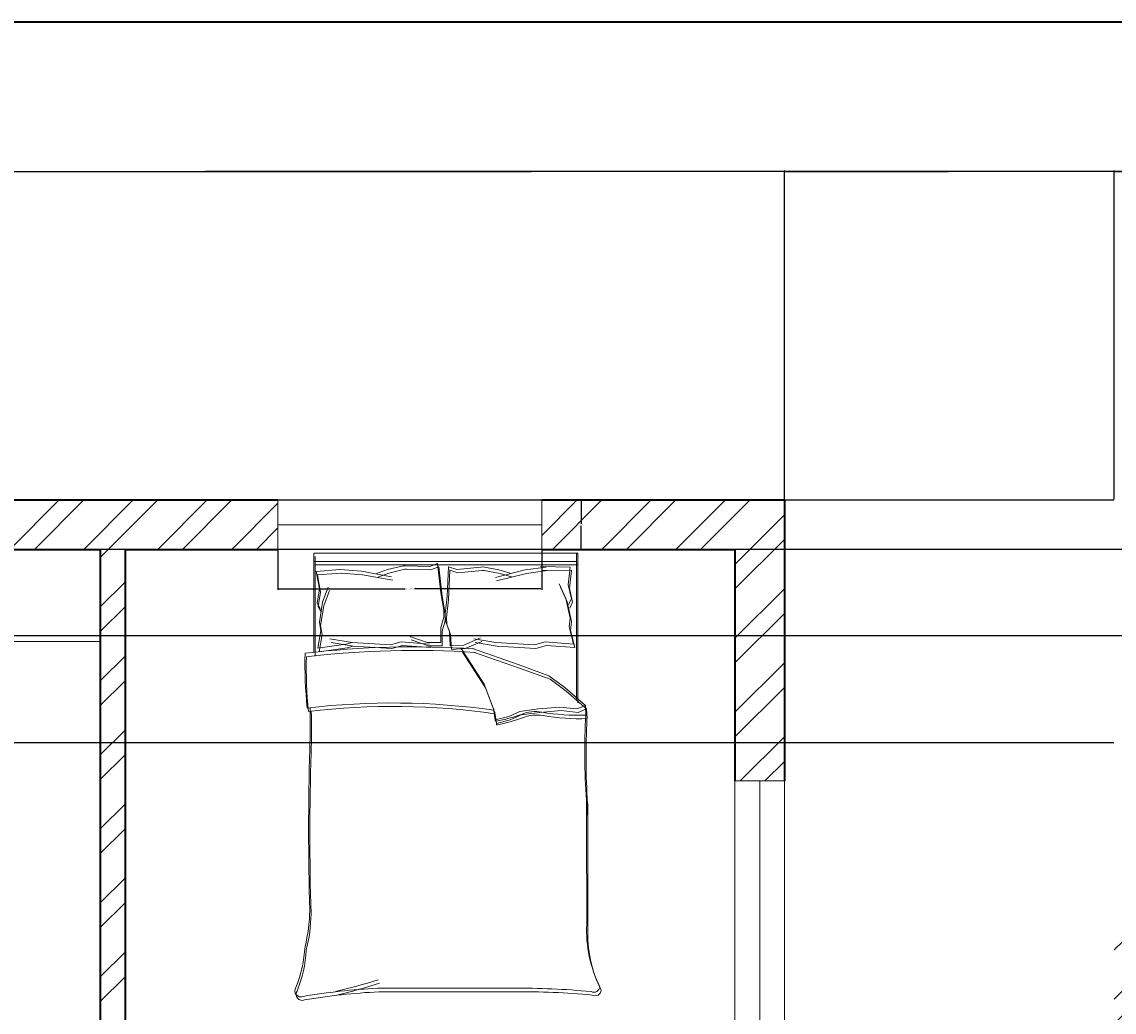
# Model space of a CAD drawing. Units: inches. Extents: x 2552 to 3217, y 1417 to 2737.
# Tile 19 of 25: x 2710 to 2909, y 2556 to 2737. Entities that reach past the tile are written whole.
import ezdxf

# ---------------------------------------------------------------- set-up
doc = ezdxf.new("R2010")
doc.units = ezdxf.units.IN
for name, color, linetype, lineweight in [('A-ANNO-DIMS', 2, 'Continuous', 18), ('A-ANNO-TTLB', 7, 'Continuous', 35), ('A-FLOR-CASE', 9, 'Continuous', 18), ('A-FURN', 8, 'Continuous', 13), ('A-GLAZ', 161, 'Continuous', 18), ('A-WALL', 7, 'Continuous', 35), ('A-WALL-PATT', 217, 'Continuous', 13)]:
    doc.layers.add(name, color=color, linetype=linetype, lineweight=lineweight)
doc.styles.get("Standard").update_dxf_attribs({"font": 'arial.ttf'})
doc.dimstyles.get("Standard").update_dxf_attribs({"dimtxt": 0.18, "dimasz": 0.18, "dimexe": 0.18, "dimexo": 0.0625, "dimgap": 0.09, "dimtad": 0, "dimtih": 1, "dimtoh": 1, "dimdec": 4, "dimzin": 0, "dimdsep": 46, "dimtxsty": 'Standard', "dimcen": 0.09, "dimadec": 0, "dimazin": 0, "dimtfac": 1, "dimtdec": 4, "dimtofl": 0, "dimtmove": 0, "dimatfit": 3, "dimfxl": 1, "dimtolj": 1, "dimtzin": 0, "dimarcsym": 0})

# ---------------------------------------------------------------- blocks, each defined once
blk = doc.blocks.new('BED-DOUBLE')
for p, q in [((3.47, 63.33), (3.47, 81.44)), ((3.47, 81.44), (51.49, 81.44)), ((3.47, 79.91), (51.27, 79.91)), ((3.48, 63.33), (3.48, 81.44)), ((3.48, 79.91), (51.27, 79.91)), ((3.7, 62.69), (3.7, 80.8)), ((3.7, 62.69), (3.7, 80.8)), ((24.54, 78.99), (25.98, 79.57)), ((24.54, 78.99), (25.98, 79.57)), ((25.98, 79.57), (26.56, 74.22)), ((25.98, 79.57), (26.56, 74.22)), ((51.27, 81.44), (51.27, 54.83)), ((51.27, 81.44), (51.27, 54.83)), ((51.49, 81.44), (51.49, 80.8)), ((51.49, 80.8), (51.49, 54.19)), ((51.49, 80.8), (51.49, 54.19)), ((3.7, 79.27), (51.49, 79.27)), ((3.7, 79.27), (51.49, 79.27)), ((3.89, 78.13), (4.47, 74.95)), ((3.89, 78.13), (4.47, 74.95)), ((3.9, 78.11), (8.18, 78.43)), ((3.9, 78.11), (8.18, 78.43)), ((4.13, 77.47), (8.41, 77.8)), ((4.13, 77.47), (8.41, 77.8)), ((8.18, 78.43), (8.28, 78.42)), ((8.18, 78.43), (8.28, 78.42)), ((8.28, 78.42), (12.11, 78.13)), ((8.28, 78.42), (12.11, 78.13)), ((8.41, 77.8), (8.51, 77.78)), ((8.41, 77.8), (8.51, 77.78)), ((8.51, 77.78), (12.34, 77.49)), ((8.51, 77.78), (12.34, 77.49)), ((12.11, 78.13), (17.6, 77.12)), ((12.11, 78.13), (17.6, 77.12)), ((14.85, 77.69), (16.88, 78.42)), ((14.85, 77.69), (16.88, 78.42)), ((15.08, 77.05), (17.11, 77.78)), ((15.08, 77.05), (17.11, 77.78)), ((16.88, 78.42), (19.77, 79.14)), ((16.88, 78.42), (19.77, 79.14)), ((17.11, 77.78), (20, 78.5)), ((17.11, 77.78), (20, 78.5)), ((19.77, 79.14), (20.09, 79.14)), ((19.77, 79.14), (20.09, 79.14)), ((20, 78.5), (20.32, 78.5)), ((20, 78.5), (20.32, 78.5)), ((20.09, 79.14), (24.54, 78.99)), ((20.09, 79.14), (24.54, 78.99)), ((20.32, 78.5), (24.77, 78.36)), ((20.32, 78.5), (24.77, 78.36)), ((24.77, 78.36), (26.21, 78.93)), ((24.77, 78.36), (26.21, 78.93)), ((26.21, 78.93), (26.79, 73.58)), ((26.21, 78.93), (26.79, 73.58)), ((27.98, 78.95), (27.73, 73.58)), ((27.98, 78.95), (27.73, 73.58)), ((28.21, 78.31), (27.96, 72.94)), ((28.21, 78.31), (27.96, 72.94)), ((29.46, 78.46), (27.98, 78.95)), ((29.46, 78.46), (27.98, 78.95)), ((29.68, 77.83), (28.21, 78.31)), ((29.68, 77.83), (28.21, 78.31)), ((33.88, 78.89), (29.46, 78.46)), ((33.88, 78.89), (29.46, 78.46)), ((34.11, 78.25), (29.68, 77.83)), ((34.11, 78.25), (29.68, 77.83)), ((34.2, 78.91), (33.88, 78.89)), ((34.2, 78.91), (33.88, 78.89)), ((34.43, 78.27), (34.11, 78.25)), ((34.43, 78.27), (34.11, 78.25)), ((37.14, 78.36), (34.2, 78.91)), ((37.14, 78.36), (34.2, 78.91)), ((37.36, 77.73), (34.43, 78.27)), ((37.36, 77.73), (34.43, 78.27)), ((41.91, 78.37), (36.49, 77.02)), ((41.91, 78.37), (36.5, 77.02)), ((42.14, 77.73), (36.72, 76.38)), ((42.14, 77.73), (36.72, 76.38)), ((39.2, 77.77), (37.14, 78.36)), ((39.2, 77.77), (37.14, 78.36)), ((39.43, 77.13), (37.36, 77.73)), ((39.43, 77.13), (37.36, 77.73)), ((45.71, 78.9), (41.91, 78.37)), ((45.71, 78.9), (41.91, 78.37)), ((45.94, 78.26), (42.14, 77.73)), ((45.94, 78.26), (42.14, 77.73)), ((50.11, 78.89), (44.71, 78.98)), ((44.71, 78.98), (45.71, 78.9)), ((50.11, 78.89), (44.71, 78.98)), ((44.71, 78.98), (45.71, 78.9)), ((50.34, 78.25), (44.94, 78.34)), ((44.94, 78.34), (45.94, 78.26)), ((50.34, 78.25), (44.94, 78.34)), ((44.94, 78.34), (45.94, 78.26)), ((50.11, 78.89), (49.73, 75.68)), ((50.11, 78.89), (49.73, 75.68)), ((50.34, 78.25), (49.96, 75.04)), ((50.34, 78.25), (49.96, 75.04)), ((4.12, 77.49), (4.7, 74.31)), ((4.12, 77.49), (4.7, 74.31)), ((12.34, 77.49), (17.83, 76.48)), ((12.34, 77.49), (17.83, 76.48)), ((49.31, 73.19), (48.13, 75.86)), ((49.31, 73.19), (48.13, 75.86)), ((49.73, 75.68), (50.33, 73.1)), ((49.73, 75.68), (50.33, 73.1)), ((4.47, 74.95), (4.04, 72.34)), ((4.47, 74.95), (4.04, 72.34)), ((4.7, 74.31), (4.27, 71.7)), ((4.7, 74.31), (4.27, 71.7)), ((5.05, 72.49), (6.06, 75.24)), ((5.05, 72.49), (6.06, 75.24)), ((5.28, 71.85), (6.29, 74.6)), ((5.28, 71.85), (6.29, 74.6)), ((26.56, 74.22), (27.14, 71.04)), ((26.56, 74.22), (27.14, 71.04)), ((26.79, 73.58), (27.37, 70.4)), ((26.79, 73.58), (27.37, 70.4)), ((27.73, 73.58), (27.35, 70.37)), ((27.73, 73.58), (27.35, 70.37)), ((49.54, 72.55), (48.36, 75.23)), ((49.54, 72.55), (48.36, 75.23)), ((49.96, 75.04), (50.56, 72.47)), ((49.96, 75.04), (50.56, 72.47)), ((4.04, 72.34), (4.62, 71.33)), ((4.04, 72.34), (4.62, 71.33)), ((4.27, 71.7), (4.85, 70.69)), ((4.27, 71.7), (4.85, 70.69)), ((4.47, 68.87), (5.05, 72.49)), ((4.47, 68.87), (5.05, 72.49)), ((4.7, 68.23), (5.28, 71.85)), ((4.7, 68.23), (5.28, 71.85)), ((27.96, 72.94), (27.58, 69.73)), ((27.96, 72.94), (27.58, 69.73)), ((50.11, 69.61), (49.31, 73.19)), ((50.11, 69.61), (49.31, 73.19)), ((50.34, 68.98), (49.54, 72.55)), ((50.34, 68.98), (49.54, 72.55)), ((50.33, 73.1), (49.81, 72.06)), ((50.33, 73.1), (49.81, 72.06)), ((50.56, 72.47), (50.04, 71.42)), ((50.56, 72.47), (50.04, 71.42)), ((27.14, 69.74), (26.56, 67.86)), ((27.14, 69.74), (26.56, 67.86)), ((27.14, 71.04), (27.14, 69.74)), ((27.14, 71.04), (27.14, 69.74)), ((27.35, 70.37), (27.44, 69.07)), ((27.35, 70.37), (27.44, 69.07)), ((27.37, 70.4), (27.37, 69.1)), ((27.37, 70.4), (27.37, 69.1)), ((27.58, 69.73), (27.66, 68.43)), ((27.58, 69.73), (27.66, 68.43)), ((49.92, 68.01), (50.11, 69.61)), ((49.92, 68.01), (50.11, 69.61)), ((4.76, 67.28), (4.47, 68.87)), ((4.76, 67.28), (4.47, 68.87)), ((4.99, 66.64), (4.7, 68.23)), ((4.99, 66.64), (4.7, 68.23)), ((26.56, 67.86), (26.56, 65.18)), ((26.56, 67.86), (26.56, 65.18)), ((27.37, 69.1), (26.79, 67.22)), ((27.37, 69.1), (26.79, 67.22)), ((27.44, 69.07), (28.13, 67.23)), ((27.44, 69.07), (28.13, 67.23)), ((27.66, 68.43), (28.36, 66.59)), ((27.66, 68.43), (28.36, 66.59)), ((50.7, 64.87), (49.92, 68.01)), ((50.7, 64.87), (49.92, 68.01)), ((50.15, 67.37), (50.34, 68.98)), ((50.15, 67.37), (50.34, 68.98)), ((4.18, 64.1), (4.76, 67.28)), ((4.18, 64.1), (4.76, 67.28)), ((4.41, 63.46), (4.99, 66.64)), ((4.41, 63.46), (4.99, 66.64)), ((6.38, 65.81), (10.41, 65.15)), ((6.38, 65.81), (10.41, 65.15)), ((24.1, 65.18), (20.96, 66.27)), ((24.1, 65.18), (20.96, 66.27)), ((24.33, 64.54), (21.19, 65.63)), ((24.33, 64.54), (21.19, 65.63)), ((26.79, 67.22), (26.79, 64.54)), ((26.79, 67.22), (26.79, 64.54)), ((28.13, 67.23), (28.3, 64.55)), ((28.13, 67.23), (28.3, 64.55)), ((28.36, 66.59), (28.53, 63.91)), ((28.36, 66.59), (28.53, 63.91)), ((30.75, 64.7), (33.82, 65.99)), ((30.75, 64.7), (33.82, 65.99)), ((32.56, 65.81), (36.6, 65.15)), ((32.56, 65.81), (36.6, 65.15)), ((50.93, 64.23), (50.15, 67.37)), ((50.93, 64.23), (50.15, 67.37)), ((9.28, 64.83), (4.18, 64.1)), ((9.28, 64.83), (4.18, 64.1)), ((9.51, 64.19), (4.41, 63.46)), ((9.51, 64.19), (4.41, 63.46)), ((6.61, 65.18), (10.64, 64.51)), ((6.61, 65.18), (10.64, 64.51)), ((10.41, 65.15), (9.28, 64.83)), ((10.41, 65.15), (9.28, 64.83)), ((10.64, 64.51), (9.51, 64.19)), ((10.64, 64.51), (9.51, 64.19)), ((10.41, 65.15), (17.42, 64.72)), ((10.41, 65.15), (17.42, 64.72)), ((10.64, 64.51), (17.65, 64.08)), ((10.64, 64.51), (17.65, 64.08)), ((17.42, 64.72), (19.38, 65.27)), ((17.42, 64.72), (19.38, 65.27)), ((17.65, 64.08), (19.61, 64.63)), ((17.65, 64.08), (19.61, 64.63)), ((19.38, 65.27), (24.52, 64.87)), ((19.38, 65.27), (24.52, 64.87)), ((19.61, 64.63), (24.74, 64.23)), ((19.61, 64.63), (24.74, 64.23)), ((26.56, 65.18), (24.1, 65.18)), ((26.56, 65.18), (24.1, 65.18)), ((26.79, 64.54), (24.33, 64.54)), ((26.79, 64.54), (24.33, 64.54)), ((28.3, 64.55), (30.75, 64.7)), ((28.3, 64.55), (30.75, 64.7)), ((28.53, 63.91), (30.98, 64.06)), ((28.53, 63.91), (30.98, 64.06)), ((30.26, 64.06), (34.45, 57.57)), ((30.26, 64.06), (34.45, 57.57)), ((30.98, 64.06), (34.05, 65.35)), ((30.98, 64.06), (34.05, 65.35)), ((40.64, 61.13), (32.31, 64.06)), ((40.64, 61.13), (32.31, 64.06)), ((32.79, 65.18), (36.82, 64.51)), ((32.79, 65.18), (36.82, 64.51)), ((36.6, 65.15), (43.61, 64.72)), ((36.6, 65.15), (43.61, 64.72)), ((36.82, 64.51), (43.83, 64.08)), ((36.82, 64.51), (43.83, 64.08)), ((43.61, 64.72), (45.57, 65.27)), ((43.61, 64.72), (45.57, 65.27)), ((43.83, 64.08), (45.79, 64.63)), ((43.83, 64.08), (45.79, 64.63)), ((45.57, 65.27), (50.7, 64.87)), ((45.57, 65.27), (50.7, 64.87)), ((45.79, 64.63), (50.93, 64.23)), ((45.79, 64.63), (50.93, 64.23)), ((30.49, 63.42), (34.68, 56.93)), ((30.49, 63.42), (34.68, 56.93)), ((40.87, 60.49), (32.53, 63.42)), ((40.87, 60.49), (32.53, 63.42)), ((46.22, 59.11), (40.64, 61.13)), ((46.22, 59.11), (40.64, 61.13)), ((46.45, 58.48), (40.87, 60.49)), ((46.45, 58.48), (40.87, 60.49)), ((49.16, 56.95), (46.22, 59.11)), ((49.16, 56.95), (46.22, 59.11)), ((49.39, 56.31), (46.45, 58.48)), ((49.39, 56.31), (46.45, 58.48)), ((34.45, 57.57), (36.15, 53.08)), ((34.45, 57.57), (36.15, 53.08)), ((34.68, 56.93), (36.38, 52.44)), ((34.68, 56.93), (36.38, 52.44)), ((52.87, 53.7), (49.16, 56.95)), ((52.87, 53.7), (49.16, 56.95)), ((53.1, 53.06), (49.39, 56.31)), ((53.1, 53.06), (49.39, 56.31)), ((51.33, 53.08), (52.87, 53.7)), ((51.33, 53.08), (52.87, 53.7)), ((52.95, 51.95), (52.87, 53.7, 3.87)), ((52.95, 51.95), (52.87, 53.7, 3.87)), ((36.15, 53.08), (36.46, 51.07)), ((36.15, 53.08), (36.46, 51.07)), ((36.38, 52.44), (36.69, 50.43)), ((36.38, 52.44), (36.69, 50.43)), ((36.46, 51.07), (38.94, 51.69)), ((36.46, 51.07), (38.94, 51.69)), ((38.94, 51.69), (40.95, 52.61)), ((38.94, 51.69), (40.95, 52.61)), ((39.17, 51.05), (41.18, 51.97)), ((39.17, 51.05), (41.18, 51.97)), ((40.95, 52.61), (44.36, 53.08)), ((40.95, 52.61), (44.36, 53.08)), ((41.18, 51.97), (44.59, 52.44)), ((41.18, 51.97), (44.59, 52.44)), ((44.36, 53.08), (48.23, 53.39)), ((44.36, 53.08), (48.23, 53.39)), ((44.59, 52.44), (48.46, 52.75)), ((44.59, 52.44), (48.46, 52.75)), ((48.23, 53.39), (51.33, 53.08)), ((48.23, 53.39), (51.33, 53.08)), ((48.46, 52.75), (51.56, 52.44)), ((48.46, 52.75), (51.56, 52.44)), ((51.56, 52.44), (53.1, 53.06)), ((51.56, 52.44), (53.1, 53.06)), ((53.18, 51.31), (53.1, 53.06, 3.87)), ((53.18, 51.31), (53.1, 53.06, 3.87)), ((36.69, 50.43), (39.17, 51.05)), ((36.69, 50.43), (39.17, 51.05)), ((15.06, 2.2), (39.68, 2.2)), ((15.06, 2.2), (39.68, 2.2)), ((15.29, 1.56), (39.91, 1.56)), ((15.29, 1.56), (39.91, 1.56))]:
    blk.add_line(p, q)
for centre, radius, start, end in [((21.36, -100.61), 164.97, 86.0865, 96.7821), ((21.36, -100.61), 164.97, 86.0865, 96.7821), ((21.59, -101.25), 164.97, 86.0865, 96.7821), ((21.59, -101.25), 164.97, 86.0865, 96.7821), ((85.16, 61.35), 83.31, 178.7218, 185.604), ((85.16, 61.35), 83.31, 178.7218, 185.604), ((85.39, 60.71), 83.31, 178.7218, 185.604), ((85.39, 60.71), 83.31, 178.7218, 185.604), ((17.76, -74.87), 129.02, 81.7845, 96.9006), ((17.76, -74.87), 129.02, 81.7845, 96.9006), ((17.98, -75.51), 129.02, 81.7845, 96.9006), ((17.98, -75.51), 129.02, 81.7845, 96.9006), ((-167.31, 50.27), 170.11, 358.4762, 1.0082), ((-167.31, 50.27), 170.11, 358.4762, 1.0082), ((-167.08, 49.63), 170.11, 358.4762, 1.0082), ((-167.08, 49.63), 170.11, 358.4762, 1.0082), ((31.15, 79.96), 29.65, 280.6617, 289.8806), ((31.15, 79.96), 29.65, 280.6617, 289.8806), ((43.74, 46.38), 6.22, 78.6608, 113.7384), ((43.74, 46.38), 6.22, 78.6608, 113.7384), ((43.97, 45.74), 6.22, 78.6608, 113.7384), ((43.97, 45.74), 6.22, 78.6608, 113.7384), ((51.33, 88.1), 36.18, 259.8763, 272.5657), ((51.33, 88.1), 36.18, 259.8763, 272.5657), ((51.56, 87.46), 36.18, 259.8763, 272.5657), ((51.56, 87.46), 36.18, 259.8763, 272.5657), ((182.27, 45.13), 129.5, 176.9791, 183.8365), ((182.27, 45.13), 129.5, 176.9791, 183.8365), ((36.64, 51), 0.185, 160.2464, 271.1377), ((36.64, 51), 0.185, 160.2464, 271.1377), ((36.86, 50.36), 0.185, 160.2464, 271.1377), ((36.86, 50.36), 0.185, 160.2464, 271.1377), ((31.38, 79.32), 29.65, 280.6617, 289.8806), ((31.38, 79.32), 29.65, 280.6617, 289.8806), ((182.49, 44.49), 129.5, 176.9791, 183.8365), ((182.49, 44.49), 129.5, 176.9791, 183.8365), ((484.82, 30.83), 482.31, 178.2277, 181.7185), ((484.82, 30.83), 482.31, 178.2277, 181.7185), ((485.05, 30.19), 482.31, 178.2277, 181.7185), ((485.05, 30.19), 482.31, 178.2277, 181.7185), ((-4508.74, 13.62), 4561.86, 0.00217, 0.28689), ((-4508.74, 13.62), 4561.86, 0.00217, 0.28689), ((-4508.51, 12.98), 4561.86, 0.00217, 0.28689), ((-4508.52, 12.98), 4561.86, 0.00217, 0.28689), ((-26.9, 16.93), 29.63, 346.0648, 358.9113), ((-26.9, 16.93), 29.63, 346.0648, 358.9113), ((-26.67, 16.29), 29.63, 346.0648, 358.9113), ((-26.67, 16.29), 29.63, 346.0648, 358.9113), ((76.16, 12.78), 23.07, 177.4714, 206.4681), ((76.16, 12.78), 23.07, 177.4714, 206.4681), ((76.39, 12.14), 23.07, 177.4714, 206.4681), ((76.39, 12.14), 23.07, 177.4714, 206.4681), ((-21.66, 11.17), 23.56, 337.9751, 356.652), ((-21.66, 11.17), 23.56, 337.9751, 356.652), ((-21.43, 10.53), 23.56, 337.9751, 356.652), ((-21.43, 10.53), 23.56, 337.9751, 356.652), ((1.09, 1.73), 1.09, 146.1736, 293.4781), ((1.09, 1.73), 1.09, 146.1736, 293.4781), ((21.43, -119.39), 121.76, 92.9958, 99.4091), ((21.43, -119.39), 121.76, 92.9958, 99.4091), ((-17.22, 105.16), 106.46, 283.3832, 287.7053), ((-17.22, 105.16), 106.46, 283.3832, 287.7053), ((-16.99, 104.52), 106.46, 283.3832, 287.7053), ((-16.99, 104.52), 106.46, 283.3832, 287.7053), ((41.15, -130.83), 133.04, 84.4998, 90.6351), ((41.15, -130.83), 133.04, 84.4998, 90.6351), ((54.41, 2.57), 1.1, 242.6588, 356.02), ((54.41, 2.57), 1.1, 242.6588, 356.02), ((1.32, 1.09), 1.09, 146.1736, 293.4781), ((1.32, 1.09), 1.09, 146.1736, 293.4781), ((21.66, -120.03), 121.76, 92.9958, 99.4091), ((21.65, -120.03), 121.76, 92.9958, 99.4091), ((41.38, -131.47), 133.04, 84.4998, 90.6351), ((41.38, -131.47), 133.04, 84.4998, 90.6351), ((54.64, 1.93), 1.1, 242.6588, 356.02), ((54.64, 1.93), 1.1, 242.6588, 356.02)]:
    blk.add_arc(centre, radius, start, end)
blk = doc.blocks.new('WIN-48-ALT')
for p, q in [((0, 0), (0, 9)), ((0, 9), (0, 4.5)), ((0, 9), (48, 9)), ((48, 4.5), (48, 9)), ((48, 9), (48, 0)), ((0, 4.5), (48, 4.5)), ((0, 0), (48, 0))]:
    blk.add_line(p, q)
blk = doc.blocks.new('*D47')
at = {"layer": 'A-ANNO-DIMS', "color": 0, "lineweight": -2, "transparency": 16777216}
for p, q in [((2756.68, 2640.45), (2756.68, 2633.13)), ((2804.68, 2640.45), (2804.68, 2633.13)), ((2756.86, 2633.31), (2779.83, 2633.31)), ((2804.5, 2633.31), (2781.52, 2633.31))]:
    blk.add_line(p, q, dxfattribs=at)
at = {"layer": 'A-ANNO-DIMS', "color": 0, "transparency": 16777216}
for points in [[(2756.86, 2633.34), (2756.86, 2633.28), (2756.68, 2633.31)], [(2804.5, 2633.34), (2804.5, 2633.28), (2804.68, 2633.31)]]:
    blk.add_solid(points, dxfattribs=at)
at = {"layer": 'Defpoints', "color": 0, "transparency": 16777216}
for p in [(2756.68, 2640.51), (2804.68, 2640.51), (2804.68, 2633.31)]:
    blk.add_point(p, dxfattribs=at)
at = {"layer": 'A-ANNO-DIMS', "color": 0, "transparency": 16777216, "insert": (2780.68, 2633.31), "char_height": 0.18, "attachment_point": 5}
blk.add_mtext('\\A1;WIN. 48 TYP.', dxfattribs=at)
blk = doc.blocks.new('*D48')
at = {"layer": 'A-ANNO-DIMS', "color": 0, "lineweight": -2, "transparency": 16777216}
for p, q in [((2804.74, 2649.51), (2812.06, 2649.51)), ((2811.88, 2649.33), (2811.88, 2645.19)), ((2811.88, 2640.69), (2811.88, 2644.83)), ((2804.74, 2640.51), (2812.06, 2640.51))]:
    blk.add_line(p, q, dxfattribs=at)
at = {"layer": 'A-ANNO-DIMS', "color": 0, "transparency": 16777216}
for points in [[(2811.85, 2649.33), (2811.91, 2649.33), (2811.88, 2649.51)], [(2811.85, 2640.69), (2811.91, 2640.69), (2811.88, 2640.51)]]:
    blk.add_solid(points, dxfattribs=at)
at = {"layer": 'Defpoints', "color": 0, "transparency": 16777216}
for p in [(2804.68, 2649.51), (2811.88, 2649.51), (2804.68, 2640.51)]:
    blk.add_point(p, dxfattribs=at)
at = {"layer": 'A-ANNO-DIMS', "color": 0, "transparency": 16777216, "insert": (2811.88, 2645.01), "char_height": 0.18, "attachment_point": 5}
blk.add_mtext('\\A1;9 TYP.', dxfattribs=at)
blk = doc.blocks.new('*D51')
at = {"layer": 'A-ANNO-DIMS', "color": 0, "lineweight": -2, "transparency": 16777216}
for p, q in [((2637.35, 2649.58), (2637.35, 2709.49)), ((2637.53, 2709.31), (2742.71, 2709.31)), ((2848.67, 2709.31), (2743.5, 2709.31)), ((2848.85, 2649.58), (2848.85, 2709.49))]:
    blk.add_line(p, q, dxfattribs=at)
at = {"layer": 'A-ANNO-DIMS', "color": 0, "transparency": 16777216}
for points in [[(2637.53, 2709.34), (2637.53, 2709.28), (2637.35, 2709.31)], [(2848.67, 2709.34), (2848.67, 2709.28), (2848.85, 2709.31)]]:
    blk.add_solid(points, dxfattribs=at)
at = {"layer": 'Defpoints', "color": 0, "transparency": 16777216}
for p in [(2848.85, 2709.31), (2637.35, 2649.51), (2848.85, 2649.51)]:
    blk.add_point(p, dxfattribs=at)
at = {"layer": 'A-ANNO-DIMS', "color": 0, "transparency": 16777216, "insert": (2743.1, 2709.31), "char_height": 0.18, "attachment_point": 5}
blk.add_mtext('\\A1;211.5', dxfattribs=at)
blk = doc.blocks.new('*D52')
at = {"layer": 'A-ANNO-DIMS', "color": 0, "lineweight": -2, "transparency": 16777216}
for p, q in [((2848.85, 2649.58), (2848.85, 2709.49)), ((2849.03, 2709.31), (2878.63, 2709.31)), ((2908.67, 2709.31), (2879.07, 2709.31)), ((2908.85, 2649.58), (2908.85, 2709.49))]:
    blk.add_line(p, q, dxfattribs=at)
at = {"layer": 'A-ANNO-DIMS', "color": 0, "transparency": 16777216}
for points in [[(2849.03, 2709.34), (2849.03, 2709.28), (2848.85, 2709.31)], [(2908.67, 2709.34), (2908.67, 2709.28), (2908.85, 2709.31)]]:
    blk.add_solid(points, dxfattribs=at)
at = {"layer": 'Defpoints', "color": 0, "transparency": 16777216}
for p in [(2908.85, 2709.31), (2848.85, 2649.51), (2908.85, 2649.51)]:
    blk.add_point(p, dxfattribs=at)
at = {"layer": 'A-ANNO-DIMS', "color": 0, "transparency": 16777216, "insert": (2878.85, 2709.31), "char_height": 0.18, "attachment_point": 5}
blk.add_mtext('\\A1;60', dxfattribs=at)
blk = doc.blocks.new('*D60')
at = {"layer": 'A-ANNO-DIMS', "color": 0, "lineweight": -2, "transparency": 16777216}
for p, q in [((2908.85, 2649.58), (2908.85, 2709.49)), ((2909.03, 2709.31), (2969.69, 2709.31)), ((3031.25, 2709.31), (2970.6, 2709.31)), ((3031.43, 2649.58), (3031.43, 2709.49))]:
    blk.add_line(p, q, dxfattribs=at)
at = {"layer": 'A-ANNO-DIMS', "color": 0, "transparency": 16777216}
for points in [[(2909.03, 2709.34), (2909.03, 2709.28), (2908.85, 2709.31)], [(3031.25, 2709.34), (3031.25, 2709.28), (3031.43, 2709.31)]]:
    blk.add_solid(points, dxfattribs=at)
at = {"layer": 'Defpoints', "color": 0, "transparency": 16777216}
for p in [(3031.43, 2709.31), (2908.85, 2649.51), (3031.43, 2649.51)]:
    blk.add_point(p, dxfattribs=at)
at = {"layer": 'A-ANNO-DIMS', "color": 0, "transparency": 16777216, "insert": (2970.14, 2709.31), "char_height": 0.18, "attachment_point": 5}
blk.add_mtext('\\A1;122.57', dxfattribs=at)
blk = doc.blocks.new('*D64')
at = {"layer": 'A-ANNO-DIMS', "color": 0, "lineweight": -2, "transparency": 16777216}
for p, q in [((2646.35, 1551.58), (2646.35, 2709.49)), ((2646.53, 2709.31), (2802.77, 2709.31)), ((2959.93, 2709.31), (2803.69, 2709.31)), ((2960.11, 1551.58), (2960.11, 2709.49))]:
    blk.add_line(p, q, dxfattribs=at)
at = {"layer": 'A-ANNO-DIMS', "color": 0, "transparency": 16777216}
for points in [[(2646.53, 2709.34), (2646.53, 2709.28), (2646.35, 2709.31)], [(2959.93, 2709.34), (2959.93, 2709.28), (2960.11, 2709.31)]]:
    blk.add_solid(points, dxfattribs=at)
at = {"layer": 'Defpoints', "color": 0, "transparency": 16777216}
for p in [(2960.11, 2709.31), (2646.35, 1551.51), (2960.11, 1551.51)]:
    blk.add_point(p, dxfattribs=at)
at = {"layer": 'A-ANNO-DIMS', "color": 0, "transparency": 16777216, "insert": (2803.23, 2709.31), "char_height": 0.18, "attachment_point": 5}
blk.add_mtext('\\A1;313.76', dxfattribs=at)
blk = doc.blocks.new('*D65')
at = {"layer": 'A-ANNO-DIMS', "color": 0, "lineweight": -2, "transparency": 16777216}
for p, q in [((2908.79, 2649.51), (2577.37, 2649.51)), ((2577.55, 2649.33), (2577.55, 2627.57)), ((2577.55, 2605.46), (2577.55, 2627.21)), ((2908.79, 2605.28), (2577.37, 2605.28))]:
    blk.add_line(p, q, dxfattribs=at)
at = {"layer": 'A-ANNO-DIMS', "color": 0, "transparency": 16777216}
for points in [[(2577.52, 2649.33), (2577.58, 2649.33), (2577.55, 2649.51)], [(2577.52, 2605.46), (2577.58, 2605.46), (2577.55, 2605.28)]]:
    blk.add_solid(points, dxfattribs=at)
at = {"layer": 'Defpoints', "color": 0, "transparency": 16777216}
for p in [(2577.55, 2649.51), (2908.85, 2649.51), (2908.85, 2605.28)]:
    blk.add_point(p, dxfattribs=at)
at = {"layer": 'A-ANNO-DIMS', "color": 0, "transparency": 16777216, "insert": (2577.55, 2627.39), "char_height": 0.18, "attachment_point": 5}
blk.add_mtext('\\A1;44.24', dxfattribs=at)
blk = doc.blocks.new('*D68')
at = {"layer": 'A-ANNO-DIMS', "color": 0, "lineweight": -2, "transparency": 16777216}
for p, q in [((2995.79, 2640.51), (2577.37, 2640.51)), ((2577.55, 2640.33), (2577.55, 2632.84)), ((2577.55, 2624.97), (2577.55, 2632.47)), ((2995.79, 2624.79), (2577.37, 2624.79))]:
    blk.add_line(p, q, dxfattribs=at)
at = {"layer": 'A-ANNO-DIMS', "color": 0, "transparency": 16777216}
for points in [[(2577.52, 2640.33), (2577.58, 2640.33), (2577.55, 2640.51)], [(2577.52, 2624.97), (2577.58, 2624.97), (2577.55, 2624.79)]]:
    blk.add_solid(points, dxfattribs=at)
at = {"layer": 'Defpoints', "color": 0, "transparency": 16777216}
for p in [(2995.85, 2640.51), (2577.55, 2624.79), (2995.85, 2624.79)]:
    blk.add_point(p, dxfattribs=at)
at = {"layer": 'A-ANNO-DIMS', "color": 0, "transparency": 16777216, "insert": (2577.55, 2632.65), "char_height": 0.18, "attachment_point": 5}
blk.add_mtext('\\A1;15.718', dxfattribs=at)

msp = doc.modelspace()

# ---------------------------------------------------------------- hatches: boundary and pattern name
at = {"layer": 'A-WALL-PATT'}
h = msp.add_hatch(dxfattribs=at)
h.set_pattern_fill('ANSI32', color=256)
h.paths.add_polyline_path([(2756.676, 2649.5125), (2637.3535, 2649.5125), (2637.3535, 2617.9626), (2641.8535, 2617.9626), (2646.3535, 2617.9626), (2646.3535, 2640.5125), (2724.3535, 2640.5125), (2724.3535, 2520.5125), (2720.299, 2520.5125), (2720.299, 2516.0125), (2733.4075, 2516.0125), (2733.4075, 2518.2213), (2733.4075, 2520.5125), (2728.8535, 2520.5125), (2728.8535, 2640.5125), (2756.676, 2640.5125)])
h.paths.add_polyline_path([(2848.8535, 2649.5125), (2804.676, 2649.5125), (2804.676, 2640.5125), (2839.8535, 2640.5125), (2839.8535, 2598.3517), (2848.8535, 2598.3517)])
h.paths.add_polyline_path([(2646.3535, 2516.0125), (2697.9593, 2516.0125), (2697.9593, 2518.2625), (2697.9593, 2520.5125), (2646.3535, 2520.5125), (2646.3535, 2581.9626), (2637.3535, 2581.9626), (2637.3535, 2364.3298), (2646.3535, 2364.3298), (2646.3535, 2387.0125), (2724.3535, 2387.0125), (2724.3535, 2267.0125), (2721.0443, 2267.0125), (2721.0443, 2262.5125), (2733.7854, 2262.5125), (2733.7854, 2264.7625), (2733.7854, 2267.0125), (2728.8535, 2267.0125), (2728.8535, 2387.0125), (2839.8535, 2387.0125), (2839.8535, 2363.8387), (2848.8535, 2363.8387), (2848.8535, 2403.7415), (2844.3535, 2403.7415), (2839.8535, 2403.7415), (2839.8535, 2396.0125), (2646.3535, 2396.0125)])
h.paths.add_polyline_path([(2848.8535, 2550.3517), (2844.3535, 2550.3517), (2839.8535, 2550.3517), (2839.8535, 2520.5125), (2801.9195, 2520.5125), (2801.9195, 2518.2625), (2801.9195, 2516.0125), (2839.8535, 2516.0125), (2839.8535, 2507.5813), (2848.8535, 2507.5813)], flags=17)
h.paths.add_polyline_path([(2848.8535, 2483.5813), (2844.3535, 2483.5813), (2839.8535, 2483.5813), (2839.8535, 2468.0125), (2773.8535, 2468.0125), (2773.8535, 2516.0125), (2778.1336, 2516.0125), (2778.1336, 2520.5125), (2766.696, 2520.5125), (2766.696, 2518.2625), (2766.696, 2516.0125), (2769.3535, 2516.0125), (2769.3535, 2463.5125), (2839.8535, 2463.5125), (2839.8535, 2431.0782), (2848.8535, 2431.0782)], flags=17)
h.paths.add_polyline_path([(2917.8535, 2569.2764), (2913.3535, 2569.2764), (2908.8535, 2569.2764), (2908.8535, 2433.001), (2917.8535, 2433.001), (2917.8535, 2516.0125), (2967.486, 2516.0125), (2967.486, 2520.5125), (2917.8535, 2520.5125)])
h.paths.add_polyline_path([(3000.3535, 2640.5125), (2995.8535, 2640.5125), (2995.8535, 2520.5125), (2990.688, 2520.5125), (2990.688, 2516.0125), (3004.0844, 2516.0125), (3004.0844, 2518.2625), (3004.0844, 2520.5125), (3000.3535, 2520.5125)])
h.paths.add_polyline_path([(3120.3535, 2561.3689), (3115.8535, 2561.3689), (3111.3535, 2561.3689), (3111.3535, 2520.5125), (3070.9814, 2520.5125), (3070.9814, 2518.2625), (3070.9814, 2516.0125), (3111.3535, 2516.0125), (3111.3535, 2505.1841), (3120.3535, 2505.1841)])
h.paths.add_polyline_path([(3120.3535, 2481.1841), (3115.8535, 2481.1841), (3111.3535, 2481.1841), (3111.3535, 2468.0125), (3045.3535, 2468.0125), (3045.3535, 2516.0125), (3048.9787, 2516.0125), (3048.9787, 2520.5125), (3036.3395, 2520.5125), (3036.3395, 2516.0125), (3040.8535, 2516.0125), (3040.8535, 2463.5125), (3111.3535, 2463.5125), (3111.3535, 2396.0125), (2917.8535, 2396.0125), (2917.8535, 2403.4124), (2913.3535, 2403.4124), (2908.8535, 2403.4124), (2908.8535, 2182.5756), (2917.8535, 2182.5756), (2917.8535, 2262.5125), (2968.001, 2262.5125), (2968.001, 2264.7625), (2968.001, 2267.0125), (2917.8535, 2267.0125), (2917.8535, 2387.0125), (3111.3535, 2387.0125), (3111.3535, 2352.2435), (3120.3535, 2352.2435)])
h.paths.add_polyline_path([(3120.3535, 2304.2435), (3115.8535, 2304.2435), (3111.3535, 2304.2435), (3111.3535, 2267.0125), (3073.8616, 2267.0125), (3073.8616, 2264.7625), (3073.8616, 2262.5125), (3111.3535, 2262.5125), (3111.3535, 2252.376), (3120.3535, 2252.376)], flags=17)
h.paths.add_polyline_path([(3120.3535, 2228.376), (3115.8535, 2228.376), (3111.3535, 2228.376), (3111.3535, 2214.5125), (3045.3535, 2214.5125), (3045.3535, 2262.5125), (3049.3096, 2262.5125), (3049.3096, 2267.0125), (3035.0125, 2267.0125), (3035.0125, 2262.5125), (3040.8535, 2262.5125), (3040.8535, 2210.0125), (3111.3535, 2210.0125), (3111.3535, 2142.5125), (2917.8535, 2142.5125), (2917.8535, 2150.2408), (2913.3535, 2150.2408), (2908.8535, 2150.2408), (2908.8535, 1924.9905), (2917.8535, 1924.9905), (2917.8535, 2009.0125), (2971.959, 2009.0125), (2971.959, 2011.2625), (2971.959, 2013.5125), (2917.8535, 2013.5125), (2917.8535, 2133.5125), (2995.8535, 2133.5125), (2995.8535, 2013.5125), (2992.1797, 2013.5125), (2992.1797, 2009.0125), (3004.3344, 2009.0125), (3004.3344, 2011.2625), (3004.3344, 2013.5125), (3000.3535, 2013.5125), (3000.3535, 2133.5125), (3111.3535, 2133.5125), (3111.3535, 2115.0291), (3120.3535, 2115.0291)])
h.paths.add_polyline_path([(3000.3535, 2387.0125), (2995.8535, 2387.0125), (2995.8535, 2267.0125), (2991.3326, 2267.0125), (2991.3326, 2262.5125), (3004.1044, 2262.5125), (3004.1044, 2264.7625), (3004.1044, 2267.0125), (3000.3535, 2267.0125)], flags=17)
h.paths.add_polyline_path([(3120.3535, 1973.2388), (3115.8535, 1973.2388), (3111.3535, 1973.2388), (3111.3535, 1961.0125), (3045.3535, 1961.0125), (3045.3535, 2009.0125), (3048.9101, 2009.0125), (3048.9101, 2013.5125), (3037.105, 2013.5125), (3037.105, 2011.2625), (3037.105, 2009.0125), (3040.8535, 2009.0125), (3040.8535, 1956.5125), (3111.3535, 1956.5125), (3111.3535, 1889.0125), (2917.8535, 1889.0125), (2917.8535, 1895.7215), (2913.3535, 1895.7215), (2908.8535, 1895.7215), (2908.8535, 1844.2217), (2917.8535, 1844.2217), (2917.8535, 1880.0125), (3111.3535, 1880.0125), (3111.3535, 1846.9541), (3120.3535, 1846.9541)])
h.paths.add_polyline_path([(3120.3535, 2067.0291), (3111.3535, 2067.0291), (3111.3535, 2013.5125), (3071.3001, 2013.5125), (3071.3001, 2009.0125), (3111.3535, 2009.0125), (3111.3535, 1997.2388), (3120.3535, 1997.2388)], flags=0)
h.paths.add_polyline_path([(3120.3535, 1798.9541), (3115.8535, 1798.9541), (3111.3535, 1798.9541), (3111.3535, 1760.0125), (3071.2497, 1760.0125), (3071.2497, 1757.7625), (3071.2497, 1755.5125), (3111.3535, 1755.5125), (3111.3535, 1746.162), (3120.3535, 1746.2478)])
h.paths.add_polyline_path([(3120.3535, 1722.2049), (3111.3535, 1722.2049), (3111.3535, 1707.5125), (3045.3535, 1707.5125), (3045.3535, 1755.5125), (3048.6624, 1755.5125), (3048.6624, 1760.0125), (3035.3703, 1760.0125), (3035.3703, 1755.5125), (3040.8535, 1755.5125), (3040.8535, 1703.0125), (3111.3535, 1703.0125), (3111.3535, 1635.5125), (2917.8535, 1635.5125), (2917.8535, 1643.1366), (2913.3535, 1643.1366), (2908.8535, 1643.1366), (2908.8535, 1626.5125), (3120.3535, 1626.5125)])
h.paths.add_polyline_path([(2917.8535, 1755.5125), (2973.2287, 1755.5125), (2973.2287, 1757.7625), (2973.2287, 1760.0125), (2917.8535, 1760.0125), (2917.8535, 1808.2217), (2913.3535, 1808.2217), (2908.8535, 1808.2217), (2908.8535, 1676.1665), (2917.8535, 1676.1665)])
h.paths.add_polyline_path([(3000.3535, 1880.0125), (2995.8535, 1880.0125), (2995.8535, 1760.0125), (2992.9329, 1760.0125), (2992.9329, 1755.5125), (3003.8766, 1755.5125), (3003.8766, 1757.7625), (3003.8766, 1760.0125), (3000.3535, 1760.0125)])
h.paths.add_polyline_path([(2848.8535, 1896.6971), (2844.3535, 1896.6971), (2839.8535, 1896.6971), (2839.8535, 1889.0125), (2646.3535, 1889.0125), (2646.3535, 2009.0125), (2700.5253, 2009.0125), (2700.5253, 2011.2625), (2700.5253, 2013.5125), (2646.3535, 2013.5125), (2646.3535, 2053.1812), (2641.8535, 2053.1812), (2637.3535, 2053.1812), (2637.3535, 1836.254), (2646.3535, 1836.254), (2646.3535, 1880.0125), (2724.3535, 1880.0125), (2724.3535, 1760.0125), (2721.2473, 1760.0125), (2721.2473, 1755.5125), (2731.9187, 1755.5125), (2731.9187, 1757.7625), (2731.9187, 1760.0125), (2728.8535, 1760.0125), (2728.8535, 1880.0125), (2839.8535, 1880.0125), (2839.8535, 1840.3813), (2848.8535, 1840.3813)])
h.paths.add_polyline_path([(2848.8535, 1792.3813), (2844.3535, 1792.3813), (2839.8535, 1792.3813), (2839.8535, 1760.0125), (2797.8845, 1760.0125), (2797.8845, 1755.5125), (2839.8535, 1755.5125), (2839.8535, 1743.3688), (2844.3535, 1743.3688), (2848.8535, 1743.3688)], flags=0)
h.paths.add_polyline_path([(2848.8535, 1719.3688), (2844.3535, 1719.3688), (2839.8535, 1719.3688), (2839.8535, 1707.5125), (2773.8535, 1707.5125), (2773.8535, 1755.5125), (2777.716, 1755.5125), (2777.716, 1760.0125), (2760.9247, 1760.0125), (2760.9247, 1757.9721), (2760.9247, 1755.5125), (2769.3535, 1755.5125), (2769.3535, 1703.0125), (2839.8535, 1703.0125), (2839.8535, 1673.0277), (2848.8535, 1672.9407)], flags=0)
h.paths.add_polyline_path([(2646.3535, 1755.5125), (2702.9171, 1755.5125), (2702.9171, 1757.7625), (2702.9171, 1760.0125), (2646.3535, 1760.0125), (2646.3535, 1800.254), (2641.8535, 1800.254), (2637.3535, 1800.254), (2637.3535, 1626.5125), (2848.8535, 1626.5125), (2848.8535, 1643.1187), (2844.3535, 1643.1187), (2839.8535, 1643.1187), (2839.8535, 1635.5125), (2646.3535, 1635.5125)])
h.paths.add_polyline_path([(2848.8535, 2148.8427), (2844.3535, 2148.8427), (2839.8535, 2148.8427), (2839.8535, 2142.5125), (2646.3535, 2142.5125), (2646.3535, 2262.5125), (2701.3562, 2262.5125), (2701.3562, 2264.7625), (2701.3562, 2267.0125), (2646.3535, 2267.0125), (2646.3535, 2328.3298), (2637.3535, 2328.3298), (2637.3535, 2089.1812), (2646.3535, 2089.1812), (2646.3535, 2133.5125), (2839.8535, 2133.5125), (2839.8535, 2097.5966), (2848.8535, 2097.5966)])
h.paths.add_polyline_path([(2728.8535, 2133.5125), (2724.3535, 2133.5125), (2724.3535, 2013.5125), (2719.6039, 2013.5125), (2719.6039, 2009.0125), (2732.5784, 2009.0125), (2732.5784, 2011.2625), (2732.5784, 2013.5125), (2728.8535, 2013.5125)])
h.paths.add_polyline_path([(2848.8535, 1970.0557), (2844.3535, 1970.0557), (2839.8535, 1970.0557), (2839.8535, 1961.0125), (2773.8535, 1961.0125), (2773.8535, 2009.0125), (2777.3388, 2009.0125), (2777.3388, 2013.5125), (2764.7681, 2013.5125), (2764.7681, 2009.0125), (2769.3535, 2009.0125), (2769.3535, 1956.5125), (2839.8535, 1956.5125), (2839.8535, 1924.7199), (2848.8535, 1924.7199)], flags=17)
h.paths.add_polyline_path([(2848.8535, 2049.5966), (2844.3535, 2049.5966), (2839.8535, 2049.5966), (2839.8535, 2013.5125), (2798.198, 2013.5125), (2798.198, 2011.2625), (2798.198, 2009.0125), (2839.8535, 2009.0125), (2839.8535, 1994.0557), (2848.8535, 1994.0557)], flags=17)
h.paths.add_polyline_path([(2848.8535, 2315.8387), (2839.8535, 2315.8387), (2839.8535, 2267.0125), (2799.3375, 2267.0125), (2799.3375, 2264.7625), (2799.3375, 2262.5125), (2839.8535, 2262.5125), (2839.8535, 2253.2843), (2848.8535, 2253.2843)], flags=17)
h.paths.add_polyline_path([(2848.8535, 2229.2843), (2839.8535, 2229.2843), (2839.8535, 2177.6936), (2848.8535, 2177.6936)], flags=17)
h.paths.add_polyline_path([(2839.8535, 2214.5125), (2773.8535, 2214.5125), (2773.8535, 2262.5125), (2777.6984, 2262.5125), (2777.6984, 2267.0125), (2763.8226, 2267.0125), (2763.8226, 2262.5125), (2769.3535, 2262.5125), (2769.3535, 2210.0125), (2839.8535, 2210.0125)], flags=17)
h.paths.add_polyline_path([(3050.32, 2520.2817), (3088.9114, 2520.2817), (3088.9114, 2538.939), (3050.32, 2538.939)], flags=9)

# ---------------------------------------------------------------- linework, layer by layer
at = {"layer": 'A-ANNO-TTLB'}
msp.add_lwpolyline([(2552.473, 2736.5692), (3216.7862, 2736.5692), (3216.7862, 1416.6914), (2552.473, 1416.6914)], close=True, dxfattribs=at)
at = {"layer": 'A-FLOR-CASE'}
msp.add_line((2662.102, 2623.7542), (2724.3535, 2623.7542), dxfattribs=at)
at = {"layer": 'A-WALL'}
for p, q in [((2637.3535, 2649.5125), (2756.676, 2649.5125)), ((2804.676, 2649.5125), (2848.8535, 2649.5125)), ((2848.8535, 2649.5125), (2848.8535, 2598.3517)), ((2646.3535, 2640.5125), (2724.3535, 2640.5125)), ((2724.3535, 2640.5125), (2724.3535, 2520.5125)), ((2728.8535, 2640.5125), (2728.8535, 2520.5125)), ((2728.8535, 2640.5125), (2756.676, 2640.5125)), ((2804.676, 2640.5125), (2839.8535, 2640.5125)), ((2839.8535, 2640.5125), (2839.8535, 2598.3517))]:
    msp.add_line(p, q, dxfattribs=at)

# ---------------------------------------------------------------- block references
at = {"layer": 'A-FURN'}
msp.add_blockref('BED-DOUBLE', (2759.753, 2558.41), dxfattribs=at)
at = {"layer": 'A-GLAZ'}
msp.add_blockref('WIN-48-ALT', (2756.676, 2640.513), dxfattribs=at)
at = {"layer": 'A-GLAZ', "extrusion": (0, 0, -1), "zscale": -1, "rotation": 90}
msp.add_blockref('WIN-48-ALT', (-2839.854, 2550.3518), dxfattribs=at)

# ---------------------------------------------------------------- dimensions: what is measured, and where the dimension line sits
at = {"layer": 'A-ANNO-DIMS'}
for base, p1, p2, override, picture, middle in [((2848.8535, 2709.3125), (2637.3535, 2649.5125), (2848.8535, 2649.5125), {"dimdec": 1, "dimlfac": 1, "dimrnd": 0, "dimzin": 0, "dimdsep": 46, "dimlunit": 2}, '*D51', (2743.1035, 2709.3125)), ((2960.1089, 2709.3125), (2646.3535, 1551.5125), (2960.1089, 1551.5125), {"dimdec": 2, "dimlfac": 1, "dimrnd": 0, "dimzin": 0, "dimdsep": 46, "dimlunit": 2}, '*D64', (2803.2312, 2709.3125)), ((2908.8535, 2709.3125), (2848.8535, 2649.5125), (2908.8535, 2649.5125), {"dimdec": 0, "dimlfac": 1, "dimrnd": 0, "dimzin": 0, "dimdsep": 46, "dimlunit": 2}, '*D52', (2878.8535, 2709.3125)), ((3031.428, 2709.3125), (2908.8535, 2649.5125), (3031.428, 2649.5125), {"dimdec": 2, "dimlfac": 1, "dimrnd": 0, "dimzin": 0, "dimdsep": 46, "dimlunit": 2}, '*D60', (2970.1408, 2709.3125))]:
    dim = msp.add_linear_dim(base=base, p1=p1, p2=p2, dimstyle='Standard', override=override, dxfattribs=at)
    dim.commit()
    dim.dimension.update_dxf_attribs({"geometry": picture, "text_midpoint": middle})
for base, p1, p2, override, picture, middle in [((2577.5535, 2649.5125), (2908.8535, 2605.2764), (2908.8535, 2649.5125), {"dimdec": 2, "dimlfac": 1, "dimrnd": 0, "dimzin": 0, "dimdsep": 46, "dimlunit": 2}, '*D65', (2577.5535, 2627.3945)), ((2577.5535, 2624.7942), (2995.8535, 2640.5125), (2995.8535, 2624.7942), {"dimdec": 3, "dimlfac": 1, "dimrnd": 0, "dimzin": 0, "dimdsep": 46, "dimlunit": 2}, '*D68', (2577.5535, 2632.6534))]:
    dim = msp.add_linear_dim(base=base, p1=p1, p2=p2, angle=90, dimstyle='Standard', override=override, dxfattribs=at)
    dim.commit()
    dim.dimension.update_dxf_attribs({"geometry": picture, "text_midpoint": middle})
dim = msp.add_linear_dim(base=(2811.876, 2649.5125), p1=(2804.676, 2640.5125), p2=(2804.676, 2649.5125), angle=90, text='<> TYP.', dimstyle='Standard', override={"dimdec": 0, "dimlfac": 1, "dimrnd": 0, "dimzin": 0, "dimdsep": 46, "dimlunit": 2}, dxfattribs=at)
dim.commit()
dim.dimension.update_dxf_attribs({"geometry": '*D48', "text_midpoint": (2811.876, 2645.0125)})
dim = msp.add_linear_dim(base=(2804.676, 2633.3125), p1=(2756.676, 2640.5125), p2=(2804.676, 2640.5125), text='WIN. <> TYP.', dimstyle='Standard', override={"dimdec": 0, "dimlfac": 1, "dimrnd": 0, "dimzin": 0, "dimdsep": 46, "dimlunit": 2}, dxfattribs=at)
dim.commit()
dim.dimension.update_dxf_attribs({"geometry": '*D47', "text_midpoint": (2780.676, 2633.3125)})

doc.saveas('drawing.dxf')
